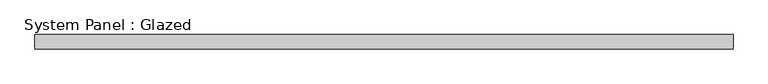
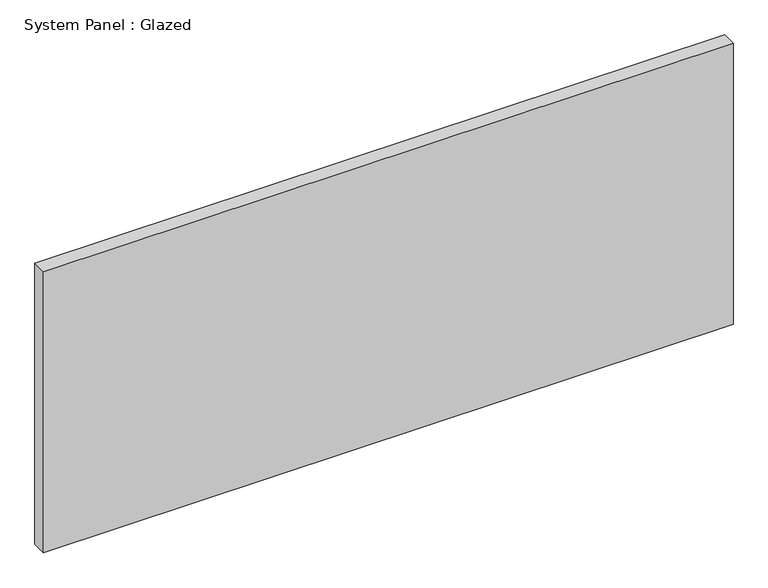
"""IFC4 building model written with IfcOpenShell, lengths in millimetres: plate geometry, System Panel : Glazed."""

from ifc_helpers import new_model, si_unit, origin, origin_with_axes, place, context, project, spatial, polyline, outline, extrude, source, transform, mapped, element, save


def system_panel_glazed_a3f6c58c(model_context):
    return source(origin(), model_context, "Body", "SweptSolid", [
        extrude(outline(polyline([(613.4099999, 19.05), (-613.4099999, 19.05), (-613.4099999, 44.45), (613.4099999, 44.45), (613.4099999, 19.05)])), origin_with_axes(), (0.0, 0.0, 1.0), 528.4534682),
    ])


if __name__ == "__main__":
    model = new_model("IFC4")
    model_context = context("Model", 3, world=origin())
    ifc_project = project(units=[si_unit("LENGTHUNIT", "METRE", prefix="MILLI")], contexts=[model_context])
    site = spatial("IfcSite", under=ifc_project)
    building = spatial("IfcBuilding", under=site)
    placement = place(None, origin())
    system_panel_glazed_shape = system_panel_glazed_a3f6c58c(model_context)
    element("IfcPlate", 1, ObjectType="System Panel : Glazed", at=placement, inside=building, context=model_context, shape_type="MappedRepresentation", body=[
        mapped(system_panel_glazed_shape, transform((0.0, 0.0, 0.0), x_axis=(1.0, 0.0, 0.0), y_axis=(0.0, 1.0, 0.0), z_axis=(0.0, 0.0, 1.0))),
    ])
    save(model, "model.ifc")

# Revit data of these elements
# Type "System Panel : Glazed"
#   Construction Type Id = "GSP4R"
#   Analytic Construction = "1/8 in Pilkington single glazing"
#   Visual Light Transmittance = 0.9
#   Solar Heat Gain Coefficient = 0.86
#   Heat Transfer Coefficient (U) = 1.18115 BTU/(h·ft²·°F)
#   Define Thermal Properties by = 1
# Element 1 (IfcPlate, "System Panel : Glazed")
#   Materials on its faces: "Glass"
# Materials
#   "Glass": class "Glass", colour RGB 0 128 192, transparency 0.75, Description = "Soda Lime Glass", Cost = 0
